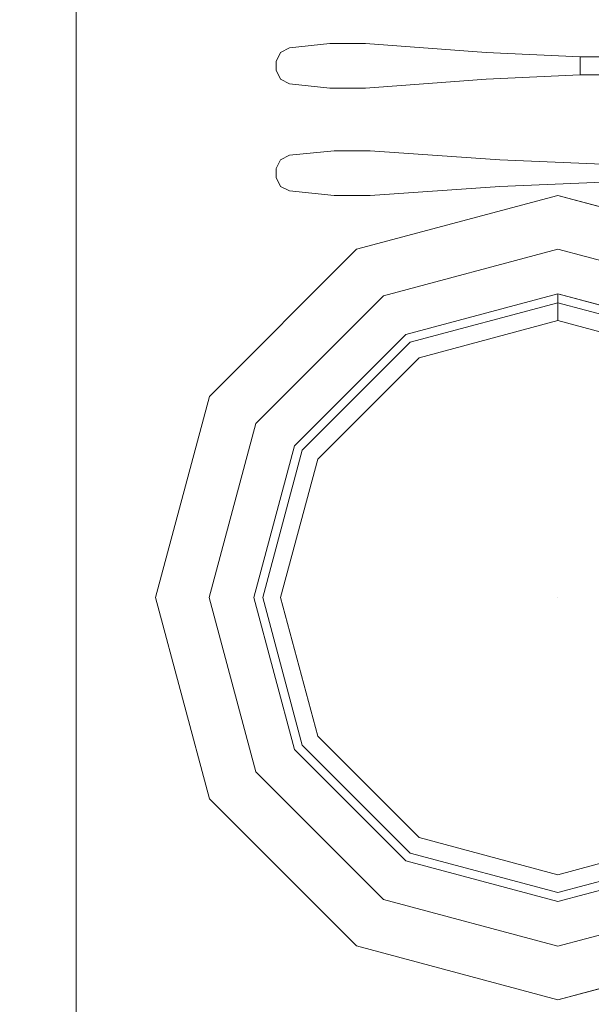
# Model space of a CAD drawing. Units: inches. Extents: x 375 to 1122, y 27 to 1069.
# Tile 95 of 155: x 705.14 to 713.02, y 863.67 to 877.23. Entities that reach past the tile are written whole.
import ezdxf

# ---------------------------------------------------------------- set-up
doc = ezdxf.new("R2010")
doc.units = ezdxf.units.IN
doc.layers.add('A-ANNO-DIMS', color=2, linetype='Continuous', lineweight=18)
doc.layers.add('Furniture', color=30, linetype='Continuous', lineweight=18)
doc.styles.get("Standard").update_dxf_attribs({"font": 'arial.ttf'})
doc.dimstyles.new('ISO-25', dxfattribs={"dimtxt": 12, "dimasz": 2.5, "dimexe": 1.5, "dimexo": 1.5, "dimtad": 1, "dimdec": 1, "dimlunit": 3, "dimtxsty": 'Standard', "dimblk": 'ARCHTICK', "dimcen": 2.5, "dimadec": 0, "dimazin": 0, "dimtfac": 1, "dimtdec": 1, "dimtmove": 0, "dimatfit": 3, "dimfxl": 1.5, "dimfxlon": 1, "dimarcsym": 0})

# ---------------------------------------------------------------- blocks, each defined once
blk = doc.blocks.new('A$C403C54AD')
blk.add_line((0.83575, 0.52421, -0.0006), (1.99923, 0.52421, -0.0006))
at = {"linetype": 'ByBlock'}
for points, invisible_edges in [([(1.72651, 0.7917, -0.01489), (1.72651, 0.69011, -0.01489), (1.72651, 0.69011, -0.01489), (1.67572, 0.77809, -0.01489)], 5), ([(1.7773, 0.77809, -0.01489), (1.72651, 0.69011, -0.01489), (1.72651, 0.69011, -0.01489), (1.72651, 0.7917, -0.01489)], 5), ([(1.67572, 0.77809, -0.01489), (1.72651, 0.69011, -0.01489), (1.72651, 0.69011, -0.01489), (1.63853, 0.74091, -0.01489)], 5), ([(1.81449, 0.74091, -0.01489), (1.72651, 0.69011, -0.01489), (1.72651, 0.69011, -0.01489), (1.7773, 0.77809, -0.01489)], 5), ([(1.60654, 0.75938, -0.00874), (1.62254, 0.75014, -0.00874), (1.60645, 0.69011, -0.00874), (1.58798, 0.69011, -0.00874)], 5), ([(1.63587, 0.74244, -0.02259), (1.60654, 0.75938, -0.01335), (1.58798, 0.69011, -0.01335), (1.62185, 0.69011, -0.02259)], 5), ([(1.83118, 0.69011, -0.02259), (1.86504, 0.69011, -0.01335), (1.84648, 0.75938, -0.01335), (1.81715, 0.74244, -0.02259)], 5), ([(1.86504, 0.69011, -0.00874), (1.84657, 0.69011, -0.00874), (1.83048, 0.75014, -0.00874), (1.84648, 0.75938, -0.00874)], 5), ([(1.62254, 0.75014, -0.00874), (1.63853, 0.74091, -0.01489), (1.62492, 0.69011, -0.01489), (1.60645, 0.69011, -0.00874)], 5), ([(1.84657, 0.69011, -0.00874), (1.8281, 0.69011, -0.01489), (1.81449, 0.74091, -0.01489), (1.83048, 0.75014, -0.00874)], 5), ([(1.63853, 0.74091, -0.01489), (1.72651, 0.69011, -0.01489), (1.72651, 0.69011, -0.01489), (1.62492, 0.69011, -0.01489)], 5), ([(1.8281, 0.69011, -0.01489), (1.72651, 0.69011, -0.01489), (1.72651, 0.69011, -0.01489), (1.81449, 0.74091, -0.01489)], 5), ([(1.82194, 0.69011, -0.03183), (1.83118, 0.69011, -0.02259), (1.81715, 0.74244, -0.02259), (1.80916, 0.73783, -0.03183)], 5), ([(1.58798, 0.69011, -0.00874), (1.60645, 0.69011, -0.00874), (1.62254, 0.63008, -0.00874), (1.60654, 0.62085, -0.00874)], 5), ([(1.62185, 0.69011, -0.02259), (1.58798, 0.69011, -0.01335), (1.60654, 0.62085, -0.01335), (1.63587, 0.63778, -0.02259)], 5), ([(1.60645, 0.69011, -0.00874), (1.62492, 0.69011, -0.01489), (1.63853, 0.63932, -0.01489), (1.62254, 0.63008, -0.00874)], 5), ([(1.63108, 0.69011, -0.03183), (1.62185, 0.69011, -0.02259), (1.63587, 0.63778, -0.02259), (1.64387, 0.6424, -0.03183)], 4), ([(1.62492, 0.69011, -0.01489), (1.72651, 0.69011, -0.01489), (1.72651, 0.69011, -0.01489), (1.63853, 0.63932, -0.01489)], 5), ([(1.63853, 0.63932, -0.01489), (1.72651, 0.69011, -0.01489), (1.72651, 0.69011, -0.01489), (1.67572, 0.60214, -0.01489)], 5), ([(1.67572, 0.60214, -0.01489), (1.72651, 0.69011, -0.01489), (1.72651, 0.69011, -0.01489), (1.72651, 0.58853, -0.01489)], 5), ([(1.72651, 0.58853, -0.01489), (1.72651, 0.69011, -0.01489), (1.72651, 0.69011, -0.01489), (1.7773, 0.60214, -0.01489)], 5), ([(1.7773, 0.60214, -0.01489), (1.72651, 0.69011, -0.01489), (1.72651, 0.69011, -0.01489), (1.81449, 0.63932, -0.01489)], 5), ([(1.81449, 0.63932, -0.01489), (1.72651, 0.69011, -0.01489), (1.72651, 0.69011, -0.01489), (1.8281, 0.69011, -0.01489)], 5), ([(1.80916, 0.6424, -0.03183), (1.81715, 0.63778, -0.02259), (1.83118, 0.69011, -0.02259), (1.82194, 0.69011, -0.03183)], 5), ([(1.83048, 0.63008, -0.00874), (1.81449, 0.63932, -0.01489), (1.8281, 0.69011, -0.01489), (1.84657, 0.69011, -0.00874)], 5), ([(1.81715, 0.63778, -0.02259), (1.84648, 0.62085, -0.01335), (1.86504, 0.69011, -0.01335), (1.83118, 0.69011, -0.02259)], 5), ([(1.84648, 0.62085, -0.00874), (1.83048, 0.63008, -0.00874), (1.84657, 0.69011, -0.00874), (1.86504, 0.69011, -0.00874)], 5), ([(1.64387, 0.6424, -0.03183), (1.63587, 0.63778, -0.02259), (1.67418, 0.59947, -0.02259), (1.6788, 0.60747, -0.03183)], 5), ([(1.77423, 0.60747, -0.03183), (1.77884, 0.59947, -0.02259), (1.81715, 0.63778, -0.02259), (1.80916, 0.6424, -0.03183)], 5), ([(1.63587, 0.63778, -0.02259), (1.60654, 0.62085, -0.01335), (1.65725, 0.57014, -0.01335), (1.67418, 0.59947, -0.02259)], 5), ([(1.62254, 0.63008, -0.00874), (1.63853, 0.63932, -0.01489), (1.67572, 0.60214, -0.01489), (1.66648, 0.58614, -0.00874)], 5), ([(1.78654, 0.58614, -0.00874), (1.7773, 0.60214, -0.01489), (1.81449, 0.63932, -0.01489), (1.83048, 0.63008, -0.00874)], 5), ([(1.77884, 0.59947, -0.02259), (1.79578, 0.57014, -0.01335), (1.84648, 0.62085, -0.01335), (1.81715, 0.63778, -0.02259)], 5), ([(1.60654, 0.62085, -0.00874), (1.62254, 0.63008, -0.00874), (1.66648, 0.58614, -0.00874), (1.65725, 0.57014, -0.00874)], 5), ([(1.79578, 0.57014, -0.00874), (1.78654, 0.58614, -0.00874), (1.83048, 0.63008, -0.00874), (1.84648, 0.62085, -0.00874)], 5), ([(1.6788, 0.60747, -0.03183), (1.67418, 0.59947, -0.02259), (1.72651, 0.58545, -0.02259), (1.72651, 0.59468, -0.03183)], 5), ([(1.72651, 0.59468, -0.03183), (1.72651, 0.58545, -0.02259), (1.77884, 0.59947, -0.02259), (1.77423, 0.60747, -0.03183)], 5), ([(1.66648, 0.58614, -0.00874), (1.67572, 0.60214, -0.01489), (1.72651, 0.58853, -0.01489), (1.72651, 0.57006, -0.00874)], 5), ([(1.72651, 0.57006, -0.00874), (1.72651, 0.58853, -0.01489), (1.7773, 0.60214, -0.01489), (1.78654, 0.58614, -0.00874)], 5), ([(1.67418, 0.59947, -0.02259), (1.65725, 0.57014, -0.01335), (1.72651, 0.55159, -0.01335), (1.72651, 0.58545, -0.02259)], 5), ([(1.72651, 0.58545, -0.02259), (1.72651, 0.55159, -0.01335), (1.79578, 0.57014, -0.01335), (1.77884, 0.59947, -0.02259)], 5), ([(1.65725, 0.57014, -0.00874), (1.66648, 0.58614, -0.00874), (1.72651, 0.57006, -0.00874), (1.72651, 0.55159, -0.00874)], 5), ([(1.72651, 0.55159, -0.00874), (1.72651, 0.57006, -0.00874), (1.78654, 0.58614, -0.00874), (1.79578, 0.57014, -0.00874)], 5)]:
    blk.add_3dface(points, dxfattribs=dict(at, invisible_edges=invisible_edges))
for points in [[(1.60654, 0.75938, -0.01335), (1.60654, 0.75938, -0.00874), (1.58798, 0.69011, -0.00874), (1.58798, 0.69011, -0.01335)], [(1.86504, 0.69011, -0.01335), (1.86504, 0.69011, -0.00874), (1.84648, 0.75938, -0.00874), (1.84648, 0.75938, -0.01335)], [(1.64387, 0.73783, -0.03183), (1.63587, 0.74244, -0.02259), (1.62185, 0.69011, -0.02259), (1.63108, 0.69011, -0.03183)], [(1.58798, 0.69011, -0.01335), (1.58798, 0.69011, -0.00874), (1.60654, 0.62085, -0.00874), (1.60654, 0.62085, -0.01335)], [(1.84648, 0.62085, -0.01335), (1.84648, 0.62085, -0.00874), (1.86504, 0.69011, -0.00874), (1.86504, 0.69011, -0.01335)], [(1.60654, 0.62085, -0.01335), (1.60654, 0.62085, -0.00874), (1.65725, 0.57014, -0.00874), (1.65725, 0.57014, -0.01335)], [(1.79578, 0.57014, -0.01335), (1.79578, 0.57014, -0.00874), (1.84648, 0.62085, -0.00874), (1.84648, 0.62085, -0.01335)], [(1.65725, 0.57014, -0.01335), (1.65725, 0.57014, -0.00874), (1.72651, 0.55159, -0.00874), (1.72651, 0.55159, -0.01335)], [(1.72651, 0.55159, -0.01335), (1.72651, 0.55159, -0.00874), (1.79578, 0.57014, -0.00874), (1.79578, 0.57014, -0.01335)]]:
    blk.add_3dface(points, dxfattribs=at)
for points in [[(1.54027, 0.69781, -0.01387), (1.54643, 0.69781, -0.01387), (1.54643, 0.70858, -0.01595), (1.54027, 0.70858, -0.01595)], [(1.54027, 0.69781, -0.01646), (1.54643, 0.69781, -0.01646), (1.54643, 0.70858, -0.01854), (1.54027, 0.70858, -0.01854)], [(1.57259, 0.62547, -0.01916), (1.57259, 0.62547, -0.0238), (1.57259, 0.61315, -0.02413), (1.57259, 0.61315, -0.01949)], [(1.58798, 0.61315, -0.01949), (1.58798, 0.61315, -0.02413), (1.58798, 0.62547, -0.0238), (1.58798, 0.62547, -0.01916)], [(1.53565, 0.62393, -0.01916), (1.53565, 0.62393, -0.0238), (1.53565, 0.61161, -0.02413), (1.53565, 0.61161, -0.01949)], [(1.55104, 0.61161, -0.01949), (1.55104, 0.61161, -0.02413), (1.55104, 0.62393, -0.0238), (1.55104, 0.62393, -0.01916)], [(1.53565, 0.61161, -0.02413), (1.53565, 0.61161, -0.01949), (1.53719, 0.59776, -0.01946), (1.53719, 0.59776, -0.02409)], [(1.5495, 0.59776, -0.02409), (1.5495, 0.59776, -0.01946), (1.55104, 0.61161, -0.01949), (1.55104, 0.61161, -0.02413)], [(1.57259, 0.61315, -0.02413), (1.57259, 0.61315, -0.01949), (1.57413, 0.59776, -0.01946), (1.57413, 0.59776, -0.02409)], [(1.58645, 0.59776, -0.02409), (1.58645, 0.59776, -0.01946), (1.58798, 0.61315, -0.01949), (1.58798, 0.61315, -0.02413)], [(1.53719, 0.59776, -0.01946), (1.53719, 0.59776, -0.02409), (1.53873, 0.59468, -0.02385), (1.53873, 0.59468, -0.01921)], [(1.54797, 0.59468, -0.01921), (1.54797, 0.59468, -0.02385), (1.5495, 0.59776, -0.02409), (1.5495, 0.59776, -0.01946)], [(1.57413, 0.59776, -0.01946), (1.57413, 0.59776, -0.02409), (1.57567, 0.59468, -0.02385), (1.57567, 0.59468, -0.01921)], [(1.58491, 0.59468, -0.01921), (1.58491, 0.59468, -0.02385), (1.58645, 0.59776, -0.02409), (1.58645, 0.59776, -0.01946)], [(1.53873, 0.59468, -0.02385), (1.53873, 0.59468, -0.01921), (1.54181, 0.59314, -0.01938), (1.54181, 0.59314, -0.02351)], [(1.54489, 0.59314, -0.02351), (1.54489, 0.59314, -0.01938), (1.54797, 0.59468, -0.01921), (1.54797, 0.59468, -0.02385)], [(1.57567, 0.59468, -0.02385), (1.57567, 0.59468, -0.01921), (1.57875, 0.59314, -0.01938), (1.57875, 0.59314, -0.02351)], [(1.58183, 0.59314, -0.02351), (1.58183, 0.59314, -0.01938), (1.58491, 0.59468, -0.01921), (1.58491, 0.59468, -0.02385)], [(1.54181, 0.59314, -0.01938), (1.54181, 0.59314, -0.02351), (1.54489, 0.59314, -0.02351), (1.54489, 0.59314, -0.01938)], [(1.57875, 0.59314, -0.01938), (1.57875, 0.59314, -0.02351), (1.58183, 0.59314, -0.02351), (1.58183, 0.59314, -0.01938)]]:
    blk.add_3dface(points)
for points, invisible_edges in [([(1.54027, 0.70858, -0.01854), (1.54027, 0.70858, -0.01595), (1.54027, 0.69781, -0.01387), (1.54027, 0.69781, -0.01646)], 5), ([(1.54643, 0.69781, -0.01646), (1.54643, 0.69781, -0.01387), (1.54643, 0.70858, -0.01595), (1.54643, 0.70858, -0.01854)], 5), ([(1.58491, 0.6701, -0.01678), (1.57567, 0.6701, -0.01678), (1.57721, 0.7055, -0.01387), (1.58337, 0.7055, -0.01387)], 1), ([(1.57721, 0.7055, -0.01387), (1.57721, 0.7055, -0.01646), (1.57567, 0.6701, -0.01986), (1.57567, 0.6701, -0.01678)], 5), ([(1.58491, 0.6701, -0.01986), (1.57567, 0.6701, -0.01986), (1.57721, 0.7055, -0.01646), (1.58337, 0.7055, -0.01646)], 1), ([(1.58491, 0.6701, -0.01678), (1.58491, 0.6701, -0.01986), (1.58337, 0.7055, -0.01646), (1.58337, 0.7055, -0.01387)], 5), ([(1.54797, 0.66549, -0.01678), (1.53873, 0.66549, -0.01678), (1.54027, 0.69781, -0.01387), (1.54643, 0.69781, -0.01387)], 1), ([(1.54027, 0.69781, -0.01387), (1.54027, 0.69781, -0.01646), (1.53873, 0.66549, -0.01986), (1.53873, 0.66549, -0.01678)], 5), ([(1.54797, 0.66549, -0.01986), (1.53873, 0.66549, -0.01986), (1.54027, 0.69781, -0.01646), (1.54643, 0.69781, -0.01646)], 1), ([(1.54797, 0.66549, -0.01678), (1.54797, 0.66549, -0.01986), (1.54643, 0.69781, -0.01646), (1.54643, 0.69781, -0.01387)], 5), ([(1.57259, 0.62547, -0.01916), (1.58798, 0.62547, -0.01916), (1.58491, 0.6701, -0.01678), (1.57567, 0.6701, -0.01678)], 5), ([(1.57259, 0.62547, -0.0238), (1.58798, 0.62547, -0.0238), (1.58491, 0.6701, -0.01986), (1.57567, 0.6701, -0.01986)], 5), ([(1.57567, 0.6701, -0.01986), (1.57567, 0.6701, -0.01678), (1.57259, 0.62547, -0.01916), (1.57259, 0.62547, -0.0238)], 1), ([(1.58798, 0.62547, -0.0238), (1.58798, 0.62547, -0.01916), (1.58491, 0.6701, -0.01678), (1.58491, 0.6701, -0.01986)], 4), ([(1.53565, 0.62393, -0.01916), (1.55104, 0.62393, -0.01916), (1.54797, 0.66549, -0.01678), (1.53873, 0.66549, -0.01678)], 5), ([(1.53565, 0.62393, -0.0238), (1.55104, 0.62393, -0.0238), (1.54797, 0.66549, -0.01986), (1.53873, 0.66549, -0.01986)], 5), ([(1.53873, 0.66549, -0.01986), (1.53873, 0.66549, -0.01678), (1.53565, 0.62393, -0.01916), (1.53565, 0.62393, -0.0238)], 1), ([(1.55104, 0.62393, -0.0238), (1.55104, 0.62393, -0.01916), (1.54797, 0.66549, -0.01678), (1.54797, 0.66549, -0.01986)], 4), ([(1.58798, 0.61315, -0.01949), (1.57259, 0.61315, -0.01949), (1.57259, 0.62547, -0.01916), (1.58798, 0.62547, -0.01916)], 5), ([(1.58798, 0.61315, -0.02413), (1.57259, 0.61315, -0.02413), (1.57259, 0.62547, -0.0238), (1.58798, 0.62547, -0.0238)], 5), ([(1.55104, 0.61161, -0.01949), (1.53565, 0.61161, -0.01949), (1.53565, 0.62393, -0.01916), (1.55104, 0.62393, -0.01916)], 5), ([(1.55104, 0.61161, -0.02413), (1.53565, 0.61161, -0.02413), (1.53565, 0.62393, -0.0238), (1.55104, 0.62393, -0.0238)], 5), ([(1.53719, 0.59776, -0.01946), (1.5495, 0.59776, -0.01946), (1.55104, 0.61161, -0.01949), (1.53565, 0.61161, -0.01949)], 5), ([(1.53719, 0.59776, -0.02409), (1.5495, 0.59776, -0.02409), (1.55104, 0.61161, -0.02413), (1.53565, 0.61161, -0.02413)], 5), ([(1.57413, 0.59776, -0.01946), (1.58645, 0.59776, -0.01946), (1.58798, 0.61315, -0.01949), (1.57259, 0.61315, -0.01949)], 5), ([(1.57413, 0.59776, -0.02409), (1.58645, 0.59776, -0.02409), (1.58798, 0.61315, -0.02413), (1.57259, 0.61315, -0.02413)], 5), ([(1.54797, 0.59468, -0.01921), (1.53873, 0.59468, -0.01921), (1.53719, 0.59776, -0.01946), (1.5495, 0.59776, -0.01946)], 5), ([(1.54797, 0.59468, -0.02385), (1.53873, 0.59468, -0.02385), (1.53719, 0.59776, -0.02409), (1.5495, 0.59776, -0.02409)], 5), ([(1.58491, 0.59468, -0.01921), (1.57567, 0.59468, -0.01921), (1.57413, 0.59776, -0.01946), (1.58645, 0.59776, -0.01946)], 5), ([(1.58491, 0.59468, -0.02385), (1.57567, 0.59468, -0.02385), (1.57413, 0.59776, -0.02409), (1.58645, 0.59776, -0.02409)], 5), ([(1.54181, 0.59314, -0.01938), (1.54489, 0.59314, -0.01938), (1.54797, 0.59468, -0.01921), (1.53873, 0.59468, -0.01921)], 4), ([(1.54181, 0.59314, -0.02351), (1.54489, 0.59314, -0.02351), (1.54797, 0.59468, -0.02385), (1.53873, 0.59468, -0.02385)], 4), ([(1.57875, 0.59314, -0.01938), (1.58183, 0.59314, -0.01938), (1.58491, 0.59468, -0.01921), (1.57567, 0.59468, -0.01921)], 4), ([(1.57875, 0.59314, -0.02351), (1.58183, 0.59314, -0.02351), (1.58491, 0.59468, -0.02385), (1.57567, 0.59468, -0.02385)], 4)]:
    blk.add_3dface(points, dxfattribs=dict(invisible_edges=invisible_edges))
blk = doc.blocks.new('_ArchTick')
at = {"color": 0, "linetype": 'ByBlock', "const_width": 0.15}
blk.add_lwpolyline([(-0.5, -0.5), (0.5, 0.5)], dxfattribs=at)
blk = doc.blocks.new('*D85')
at = {"layer": 'A-ANNO-DIMS', "color": 0, "lineweight": -2, "transparency": 16777216}
for p, q in [((401.507, 868.528), (398.507, 868.528)), ((400.007, 814.528), (400.007, 868.528)), ((401.507, 814.528), (398.507, 814.528))]:
    blk.add_line(p, q, dxfattribs=at)
at = {"layer": 'Defpoints', "color": 0, "transparency": 16777216}
for p in [(400.007, 868.528), (845.007, 868.528), (845.007, 814.528)]:
    blk.add_point(p, dxfattribs=at)
at = {"layer": 'A-ANNO-DIMS', "color": 0, "lineweight": -2, "transparency": 16777216, "xscale": 2.5, "yscale": 2.5, "zscale": 2.5}
for p, rotation in [((400.007, 868.528), 90), ((400.007, 814.528), 270)]:
    blk.add_blockref('_ArchTick', p, dxfattribs=dict(at, rotation=rotation))
at = {"layer": 'A-ANNO-DIMS', "color": 0, "transparency": 16777216, "insert": (393.255, 841.528), "char_height": 12, "attachment_point": 5, "rotation": 90}
blk.add_mtext('4\'-6"', dxfattribs=at)

msp = doc.modelspace()

# ---------------------------------------------------------------- block references
at = {"layer": 'Furniture', "xscale": 39.9918517141215, "yscale": 39.9918517141215, "zscale": 39.9918517141215, "rotation": 270}
msp.add_blockref('A$C403C54AD', (684.955, 938.316, 0.024), dxfattribs=at)

# ---------------------------------------------------------------- dimensions: what is measured, and where the dimension line sits
at = {"layer": 'A-ANNO-DIMS'}
dim = msp.add_linear_dim(base=(400.007, 868.528), p1=(845.007, 814.528), p2=(845.007, 868.528), angle=90, dimstyle='ISO-25', override={"dimdec": 1, "dimlfac": 1, "dimrnd": 0, "dimzin": 1, "dimdsep": 46, "dimlunit": 4, "dimfrac": 2}, dxfattribs=at)
dim.commit()
dim.dimension.update_dxf_attribs({"geometry": '*D85', "text_midpoint": (393.255, 841.528)})

doc.saveas('drawing.dxf')
